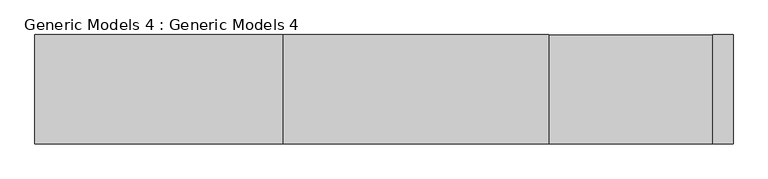
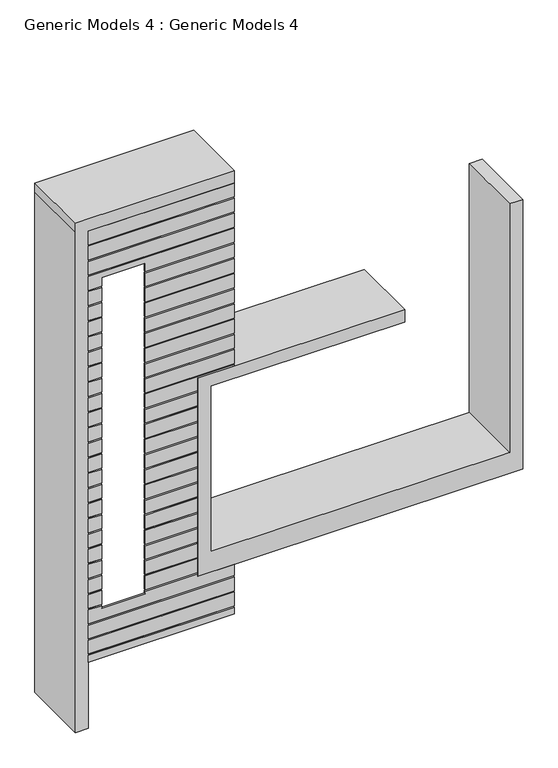
"""IFC4 building model written with IfcOpenShell, lengths in millimetres: proxy geometry, Generic Models 4 : Generic Models 4."""

from ifc_helpers import new_model, si_unit, frame, origin, place, context, project, spatial, polyline, outline, extrude, source, transform, mapped, element, save


def generic_models_4_generic_models_4_1a732ec2(model_context):
    return source(origin(), model_context, "Body", "SweptSolid", [
        extrude(outline(polyline([(-19482.368705, -12114.7027976), (-16942.368705, -12114.7027976), (-16942.368705, -12140.1027976), (-19482.368705, -12140.1027976), (-19482.368705, -12114.7027976)])), frame((0.0, 0.0, 11198.4492635), z_axis=(0.0, 0.0, 1.0), x_axis=(1.0, 0.0, 0.0)), (0.0, 0.0, 1.0), 254.0),
        extrude(outline(polyline([(-19482.368705, -12114.7027976), (-16942.368705, -12114.7027976), (-16942.368705, -12140.1027976), (-19482.368705, -12140.1027976), (-19482.368705, -12114.7027976)])), frame((0.0, 0.0, 10919.0492635), z_axis=(0.0, 0.0, 1.0), x_axis=(1.0, 0.0, 0.0)), (0.0, 0.0, 1.0), 254.0),
        extrude(outline(polyline([(-19482.368705, -12114.7027976), (-16942.368705, -12114.7027976), (-16942.368705, -12140.1027976), (-19482.368705, -12140.1027976), (-19482.368705, -12114.7027976)])), frame((0.0, 0.0, 10639.6492635), z_axis=(0.0, 0.0, 1.0), x_axis=(1.0, 0.0, 0.0)), (0.0, 0.0, 1.0), 254.0),
        extrude(outline(polyline([(10614.2492635, -19482.368705), (10360.2492635, -19482.368705), (10360.2492635, -19253.768705), (10515.6, -19253.768705), (10515.6, -18491.768705), (10360.2492635, -18491.768705), (10360.2492635, -16942.368705), (10614.2492635, -16942.368705), (10614.2492635, -19482.368705)])), frame((0.0, -12140.1027976, 0.0), z_axis=(0.0, 1.0, 0.0), x_axis=(0.0, 0.0, 1.0)), (0.0, 0.0, 1.0), 25.4),
        extrude(outline(polyline([(-18491.768705, -12114.7027976), (-16942.368705, -12114.7027976), (-16942.368705, -12140.1027976), (-18491.768705, -12140.1027976), (-18491.768705, -12114.7027976)])), frame((0.0, 0.0, 10080.8492635), z_axis=(0.0, 0.0, 1.0), x_axis=(1.0, 0.0, 0.0)), (0.0, 0.0, 1.0), 254.0),
        extrude(outline(polyline([(-19482.368705, -12114.7027976), (-19253.768705, -12114.7027976), (-19253.768705, -12140.1027976), (-19482.368705, -12140.1027976), (-19482.368705, -12114.7027976)])), frame((0.0, 0.0, 10080.8492635), z_axis=(0.0, 0.0, 1.0), x_axis=(1.0, 0.0, 0.0)), (0.0, 0.0, 1.0), 254.0),
        extrude(outline(polyline([(-18491.768705, -12114.7027976), (-16942.368705, -12114.7027976), (-16942.368705, -12140.1027976), (-18491.768705, -12140.1027976), (-18491.768705, -12114.7027976)])), frame((0.0, 0.0, 9801.4492635), z_axis=(0.0, 0.0, 1.0), x_axis=(1.0, 0.0, 0.0)), (0.0, 0.0, 1.0), 254.0),
        extrude(outline(polyline([(-19482.368705, -12114.7027976), (-19253.768705, -12114.7027976), (-19253.768705, -12140.1027976), (-19482.368705, -12140.1027976), (-19482.368705, -12114.7027976)])), frame((0.0, 0.0, 9801.4492635), z_axis=(0.0, 0.0, 1.0), x_axis=(1.0, 0.0, 0.0)), (0.0, 0.0, 1.0), 254.0),
        extrude(outline(polyline([(-18491.768705, -12114.7027976), (-16942.368705, -12114.7027976), (-16942.368705, -12140.1027976), (-18491.768705, -12140.1027976), (-18491.768705, -12114.7027976)])), frame((0.0, 0.0, 9522.0492635), z_axis=(0.0, 0.0, 1.0), x_axis=(1.0, 0.0, 0.0)), (0.0, 0.0, 1.0), 254.0),
        extrude(outline(polyline([(-19482.368705, -12114.7027976), (-19253.768705, -12114.7027976), (-19253.768705, -12140.1027976), (-19482.368705, -12140.1027976), (-19482.368705, -12114.7027976)])), frame((0.0, 0.0, 9522.0492635), z_axis=(0.0, 0.0, 1.0), x_axis=(1.0, 0.0, 0.0)), (0.0, 0.0, 1.0), 254.0),
        extrude(outline(polyline([(-18491.768705, -12114.7027976), (-16942.368705, -12114.7027976), (-16942.368705, -12140.1027976), (-18491.768705, -12140.1027976), (-18491.768705, -12114.7027976)])), frame((0.0, 0.0, 9242.6492635), z_axis=(0.0, 0.0, 1.0), x_axis=(1.0, 0.0, 0.0)), (0.0, 0.0, 1.0), 254.0),
        extrude(outline(polyline([(-19482.368705, -12114.7027976), (-19253.768705, -12114.7027976), (-19253.768705, -12140.1027976), (-19482.368705, -12140.1027976), (-19482.368705, -12114.7027976)])), frame((0.0, 0.0, 9242.6492635), z_axis=(0.0, 0.0, 1.0), x_axis=(1.0, 0.0, 0.0)), (0.0, 0.0, 1.0), 254.0),
        extrude(outline(polyline([(-18491.768705, -12114.7027976), (-16942.368705, -12114.7027976), (-16942.368705, -12140.1027976), (-18491.768705, -12140.1027976), (-18491.768705, -12114.7027976)])), frame((0.0, 0.0, 8963.2492635), z_axis=(0.0, 0.0, 1.0), x_axis=(1.0, 0.0, 0.0)), (0.0, 0.0, 1.0), 254.0),
        extrude(outline(polyline([(-19482.368705, -12114.7027976), (-19253.768705, -12114.7027976), (-19253.768705, -12140.1027976), (-19482.368705, -12140.1027976), (-19482.368705, -12114.7027976)])), frame((0.0, 0.0, 8963.2492635), z_axis=(0.0, 0.0, 1.0), x_axis=(1.0, 0.0, 0.0)), (0.0, 0.0, 1.0), 254.0),
        extrude(outline(polyline([(-18491.768705, -12114.7027976), (-16942.368705, -12114.7027976), (-16942.368705, -12140.1027976), (-18491.768705, -12140.1027976), (-18491.768705, -12114.7027976)])), frame((0.0, 0.0, 8683.8492635), z_axis=(0.0, 0.0, 1.0), x_axis=(1.0, 0.0, 0.0)), (0.0, 0.0, 1.0), 254.0),
        extrude(outline(polyline([(-19482.368705, -12114.7027976), (-19253.768705, -12114.7027976), (-19253.768705, -12140.1027976), (-19482.368705, -12140.1027976), (-19482.368705, -12114.7027976)])), frame((0.0, 0.0, 8683.8492635), z_axis=(0.0, 0.0, 1.0), x_axis=(1.0, 0.0, 0.0)), (0.0, 0.0, 1.0), 254.0),
        extrude(outline(polyline([(-18491.768705, -12114.7027976), (-16942.368705, -12114.7027976), (-16942.368705, -12140.1027976), (-18491.768705, -12140.1027976), (-18491.768705, -12114.7027976)])), frame((0.0, 0.0, 8404.4492635), z_axis=(0.0, 0.0, 1.0), x_axis=(1.0, 0.0, 0.0)), (0.0, 0.0, 1.0), 254.0),
        extrude(outline(polyline([(-19482.368705, -12114.7027976), (-19253.768705, -12114.7027976), (-19253.768705, -12140.1027976), (-19482.368705, -12140.1027976), (-19482.368705, -12114.7027976)])), frame((0.0, 0.0, 8404.4492635), z_axis=(0.0, 0.0, 1.0), x_axis=(1.0, 0.0, 0.0)), (0.0, 0.0, 1.0), 254.0),
        extrude(outline(polyline([(-18491.768705, -12114.7027976), (-16942.368705, -12114.7027976), (-16942.368705, -12140.1027976), (-18491.768705, -12140.1027976), (-18491.768705, -12114.7027976)])), frame((0.0, 0.0, 8125.0492635), z_axis=(0.0, 0.0, 1.0), x_axis=(1.0, 0.0, 0.0)), (0.0, 0.0, 1.0), 254.0),
        extrude(outline(polyline([(-19482.368705, -12114.7027976), (-19253.768705, -12114.7027976), (-19253.768705, -12140.1027976), (-19482.368705, -12140.1027976), (-19482.368705, -12114.7027976)])), frame((0.0, 0.0, 8125.0492635), z_axis=(0.0, 0.0, 1.0), x_axis=(1.0, 0.0, 0.0)), (0.0, 0.0, 1.0), 254.0),
        extrude(outline(polyline([(8099.6492635, -18491.768705), (7845.6492635, -18491.768705), (7845.6492635, -17577.368705), (8077.2, -17577.368705), (8077.2, -16942.368705), (8099.6492635, -16942.368705), (8099.6492635, -18491.768705)])), frame((0.0, -12140.1027976, 0.0), z_axis=(0.0, 1.0, 0.0), x_axis=(0.0, 0.0, 1.0)), (0.0, 0.0, 1.0), 25.4),
        extrude(outline(polyline([(-19482.368705, -12114.7027976), (-19253.768705, -12114.7027976), (-19253.768705, -12140.1027976), (-19482.368705, -12140.1027976), (-19482.368705, -12114.7027976)])), frame((0.0, 0.0, 7845.6492635), z_axis=(0.0, 0.0, 1.0), x_axis=(1.0, 0.0, 0.0)), (0.0, 0.0, 1.0), 254.0),
        extrude(outline(polyline([(-18491.768705, -12114.7027976), (-17577.368705, -12114.7027976), (-17577.368705, -12140.1027976), (-18491.768705, -12140.1027976), (-18491.768705, -12114.7027976)])), frame((0.0, 0.0, 7566.2492635), z_axis=(0.0, 0.0, 1.0), x_axis=(1.0, 0.0, 0.0)), (0.0, 0.0, 1.0), 254.0),
        extrude(outline(polyline([(-19482.368705, -12114.7027976), (-19253.768705, -12114.7027976), (-19253.768705, -12140.1027976), (-19482.368705, -12140.1027976), (-19482.368705, -12114.7027976)])), frame((0.0, 0.0, 7566.2492635), z_axis=(0.0, 0.0, 1.0), x_axis=(1.0, 0.0, 0.0)), (0.0, 0.0, 1.0), 254.0),
        extrude(outline(polyline([(-18491.768705, -12114.7027976), (-17577.368705, -12114.7027976), (-17577.368705, -12140.1027976), (-18491.768705, -12140.1027976), (-18491.768705, -12114.7027976)])), frame((0.0, 0.0, 7286.8492635), z_axis=(0.0, 0.0, 1.0), x_axis=(1.0, 0.0, 0.0)), (0.0, 0.0, 1.0), 254.0),
        extrude(outline(polyline([(-19482.368705, -12114.7027976), (-19253.768705, -12114.7027976), (-19253.768705, -12140.1027976), (-19482.368705, -12140.1027976), (-19482.368705, -12114.7027976)])), frame((0.0, 0.0, 7286.8492635), z_axis=(0.0, 0.0, 1.0), x_axis=(1.0, 0.0, 0.0)), (0.0, 0.0, 1.0), 254.0),
        extrude(outline(polyline([(-18491.768705, -12114.7027976), (-17577.368705, -12114.7027976), (-17577.368705, -12140.1027976), (-18491.768705, -12140.1027976), (-18491.768705, -12114.7027976)])), frame((0.0, 0.0, 7007.4492635), z_axis=(0.0, 0.0, 1.0), x_axis=(1.0, 0.0, 0.0)), (0.0, 0.0, 1.0), 254.0),
        extrude(outline(polyline([(-19482.368705, -12114.7027976), (-19253.768705, -12114.7027976), (-19253.768705, -12140.1027976), (-19482.368705, -12140.1027976), (-19482.368705, -12114.7027976)])), frame((0.0, 0.0, 7007.4492635), z_axis=(0.0, 0.0, 1.0), x_axis=(1.0, 0.0, 0.0)), (0.0, 0.0, 1.0), 254.0),
        extrude(outline(polyline([(-18491.768705, -12114.7027976), (-17577.368705, -12114.7027976), (-17577.368705, -12140.1027976), (-18491.768705, -12140.1027976), (-18491.768705, -12114.7027976)])), frame((0.0, 0.0, 6728.0492635), z_axis=(0.0, 0.0, 1.0), x_axis=(1.0, 0.0, 0.0)), (0.0, 0.0, 1.0), 254.0),
        extrude(outline(polyline([(-19482.368705, -12114.7027976), (-19253.768705, -12114.7027976), (-19253.768705, -12140.1027976), (-19482.368705, -12140.1027976), (-19482.368705, -12114.7027976)])), frame((0.0, 0.0, 6728.0492635), z_axis=(0.0, 0.0, 1.0), x_axis=(1.0, 0.0, 0.0)), (0.0, 0.0, 1.0), 254.0),
        extrude(outline(polyline([(-18491.768705, -12114.7027976), (-17577.368705, -12114.7027976), (-17577.368705, -12140.1027976), (-18491.768705, -12140.1027976), (-18491.768705, -12114.7027976)])), frame((0.0, 0.0, 6448.6492635), z_axis=(0.0, 0.0, 1.0), x_axis=(1.0, 0.0, 0.0)), (0.0, 0.0, 1.0), 254.0),
        extrude(outline(polyline([(-19482.368705, -12114.7027976), (-19253.768705, -12114.7027976), (-19253.768705, -12140.1027976), (-19482.368705, -12140.1027976), (-19482.368705, -12114.7027976)])), frame((0.0, 0.0, 6448.6492635), z_axis=(0.0, 0.0, 1.0), x_axis=(1.0, 0.0, 0.0)), (0.0, 0.0, 1.0), 254.0),
        extrude(outline(polyline([(-18491.768705, -12114.7027976), (-17577.368705, -12114.7027976), (-17577.368705, -12140.1027976), (-18491.768705, -12140.1027976), (-18491.768705, -12114.7027976)])), frame((0.0, 0.0, 6169.2492635), z_axis=(0.0, 0.0, 1.0), x_axis=(1.0, 0.0, 0.0)), (0.0, 0.0, 1.0), 254.0),
        extrude(outline(polyline([(-19482.368705, -12114.7027976), (-19253.768705, -12114.7027976), (-19253.768705, -12140.1027976), (-19482.368705, -12140.1027976), (-19482.368705, -12114.7027976)])), frame((0.0, 0.0, 6169.2492635), z_axis=(0.0, 0.0, 1.0), x_axis=(1.0, 0.0, 0.0)), (0.0, 0.0, 1.0), 254.0),
        extrude(outline(polyline([(-18491.768705, -12114.7027976), (-17577.368705, -12114.7027976), (-17577.368705, -12140.1027976), (-18491.768705, -12140.1027976), (-18491.768705, -12114.7027976)])), frame((0.0, 0.0, 5889.8492635), z_axis=(0.0, 0.0, 1.0), x_axis=(1.0, 0.0, 0.0)), (0.0, 0.0, 1.0), 254.0),
        extrude(outline(polyline([(-19482.368705, -12114.7027976), (-19253.768705, -12114.7027976), (-19253.768705, -12140.1027976), (-19482.368705, -12140.1027976), (-19482.368705, -12114.7027976)])), frame((0.0, 0.0, 5889.8492635), z_axis=(0.0, 0.0, 1.0), x_axis=(1.0, 0.0, 0.0)), (0.0, 0.0, 1.0), 254.0),
        extrude(outline(polyline([(-18491.768705, -12114.7027976), (-17577.368705, -12114.7027976), (-17577.368705, -12140.1027976), (-18491.768705, -12140.1027976), (-18491.768705, -12114.7027976)])), frame((0.0, 0.0, 5610.4492635), z_axis=(0.0, 0.0, 1.0), x_axis=(1.0, 0.0, 0.0)), (0.0, 0.0, 1.0), 254.0),
        extrude(outline(polyline([(-19482.368705, -12114.7027976), (-19253.768705, -12114.7027976), (-19253.768705, -12140.1027976), (-19482.368705, -12140.1027976), (-19482.368705, -12114.7027976)])), frame((0.0, 0.0, 5610.4492635), z_axis=(0.0, 0.0, 1.0), x_axis=(1.0, 0.0, 0.0)), (0.0, 0.0, 1.0), 254.0),
        extrude(outline(polyline([(-18491.768705, -12114.7027976), (-17577.368705, -12114.7027976), (-17577.368705, -12140.1027976), (-18491.768705, -12140.1027976), (-18491.768705, -12114.7027976)])), frame((0.0, 0.0, 5331.0492635), z_axis=(0.0, 0.0, 1.0), x_axis=(1.0, 0.0, 0.0)), (0.0, 0.0, 1.0), 254.0),
        extrude(outline(polyline([(-19482.368705, -12114.7027976), (-19253.768705, -12114.7027976), (-19253.768705, -12140.1027976), (-19482.368705, -12140.1027976), (-19482.368705, -12114.7027976)])), frame((0.0, 0.0, 5331.0492635), z_axis=(0.0, 0.0, 1.0), x_axis=(1.0, 0.0, 0.0)), (0.0, 0.0, 1.0), 254.0),
        extrude(outline(polyline([(-18491.768705, -12114.7027976), (-17577.368705, -12114.7027976), (-17577.368705, -12140.1027976), (-18491.768705, -12140.1027976), (-18491.768705, -12114.7027976)])), frame((0.0, 0.0, 5051.6492635), z_axis=(0.0, 0.0, 1.0), x_axis=(1.0, 0.0, 0.0)), (0.0, 0.0, 1.0), 254.0),
        extrude(outline(polyline([(-19482.368705, -12114.7027976), (-19253.768705, -12114.7027976), (-19253.768705, -12140.1027976), (-19482.368705, -12140.1027976), (-19482.368705, -12114.7027976)])), frame((0.0, 0.0, 5051.6492635), z_axis=(0.0, 0.0, 1.0), x_axis=(1.0, 0.0, 0.0)), (0.0, 0.0, 1.0), 254.0),
        extrude(outline(polyline([(-18491.768705, -12114.7027976), (-17577.368705, -12114.7027976), (-17577.368705, -12140.1027976), (-18491.768705, -12140.1027976), (-18491.768705, -12114.7027976)])), frame((0.0, 0.0, 4772.2492635), z_axis=(0.0, 0.0, 1.0), x_axis=(1.0, 0.0, 0.0)), (0.0, 0.0, 1.0), 254.0),
        extrude(outline(polyline([(-19482.368705, -12114.7027976), (-19253.768705, -12114.7027976), (-19253.768705, -12140.1027976), (-19482.368705, -12140.1027976), (-19482.368705, -12114.7027976)])), frame((0.0, 0.0, 4772.2492635), z_axis=(0.0, 0.0, 1.0), x_axis=(1.0, 0.0, 0.0)), (0.0, 0.0, 1.0), 254.0),
        extrude(outline(polyline([(-18491.768705, -12114.7027976), (-17577.368705, -12114.7027976), (-17577.368705, -12140.1027976), (-18491.768705, -12140.1027976), (-18491.768705, -12114.7027976)])), frame((0.0, 0.0, 4492.8492635), z_axis=(0.0, 0.0, 1.0), x_axis=(1.0, 0.0, 0.0)), (0.0, 0.0, 1.0), 254.0),
        extrude(outline(polyline([(-19482.368705, -12114.7027976), (-19253.768705, -12114.7027976), (-19253.768705, -12140.1027976), (-19482.368705, -12140.1027976), (-19482.368705, -12114.7027976)])), frame((0.0, 0.0, 4492.8492635), z_axis=(0.0, 0.0, 1.0), x_axis=(1.0, 0.0, 0.0)), (0.0, 0.0, 1.0), 254.0),
        extrude(outline(polyline([(4467.4492635, -18491.768705), (4419.6, -18491.768705), (4419.6, -19253.768705), (4467.4492635, -19253.768705), (4467.4492635, -19482.368705), (4213.4492635, -19482.368705), (4213.4492635, -16942.368705), (4419.6, -16942.368705), (4419.6, -17577.368705), (4467.4492635, -17577.368705), (4467.4492635, -18491.768705)])), frame((0.0, -12140.1027976, 0.0), z_axis=(0.0, 1.0, 0.0), x_axis=(0.0, 0.0, 1.0)), (0.0, 0.0, 1.0), 25.4),
        extrude(outline(polyline([(-19482.368705, -12114.7027976), (-16942.368705, -12114.7027976), (-16942.368705, -12140.1027976), (-19482.368705, -12140.1027976), (-19482.368705, -12114.7027976)])), frame((0.0, 0.0, 3934.0492635), z_axis=(0.0, 0.0, 1.0), x_axis=(1.0, 0.0, 0.0)), (0.0, 0.0, 1.0), 254.0),
        extrude(outline(polyline([(-19482.368705, -12114.7027976), (-16942.368705, -12114.7027976), (-16942.368705, -12140.1027976), (-19482.368705, -12140.1027976), (-19482.368705, -12114.7027976)])), frame((0.0, 0.0, 3654.6492635), z_axis=(0.0, 0.0, 1.0), x_axis=(1.0, 0.0, 0.0)), (0.0, 0.0, 1.0), 254.0),
        extrude(outline(polyline([(-19482.368705, -12114.7027976), (-16942.368705, -12114.7027976), (-16942.368705, -12140.1027976), (-19482.368705, -12140.1027976), (-19482.368705, -12114.7027976)])), frame((0.0, 0.0, 3505.2), z_axis=(0.0, 0.0, 1.0), x_axis=(1.0, 0.0, 0.0)), (0.0, 0.0, 1.0), 124.0492635),
        extrude(outline(polyline([(4419.6, -11913.168705), (4800.6, -11913.168705), (9386.2446878, -11913.168705), (9386.2446878, -12141.768705), (4800.6, -12141.768705), (4800.6, -17348.768705), (7848.6, -17348.768705), (7848.6, -13970.568705), (8077.2, -13970.568705), (8077.2, -17577.368705), (7848.6, -17577.368705), (4800.6, -17577.368705), (4419.6, -17577.368705), (4419.6, -11913.168705)])), frame((0.0, -12140.1027976, 0.0), z_axis=(0.0, 1.0, 0.0), x_axis=(0.0, 0.0, 1.0)), (0.0, 0.0, 1.0), 1219.2),
        extrude(outline(polyline([(11452.4492635, -19482.368705), (11452.4492635, -16942.368705), (11681.0492635, -16942.368705), (11681.0492635, -19710.968705), (11506.2, -19710.968705), (2286.0, -19710.968705), (2286.0, -19482.368705), (11452.4492635, -19482.368705)])), frame((0.0, -12140.1027976, 0.0), z_axis=(0.0, 1.0, 0.0), x_axis=(0.0, 0.0, 1.0)), (0.0, 0.0, 1.0), 1219.2),
    ])


if __name__ == "__main__":
    model = new_model("IFC4")
    model_context = context("Model", 3, world=origin())
    ifc_project = project(units=[si_unit("LENGTHUNIT", "METRE", prefix="MILLI")], contexts=[model_context])
    site = spatial("IfcSite", under=ifc_project)
    building = spatial("IfcBuilding", under=site)
    placement = place(None, origin())
    generic_models_4_generic_models_4_shape = generic_models_4_generic_models_4_1a732ec2(model_context)
    element("IfcBuildingElementProxy", 1, Name="Generic Models 4 : Generic Models 4", ObjectType="Generic Models 4 : Generic Models 4", at=placement, inside=building, context=model_context, shape_type="MappedRepresentation", body=[
        mapped(generic_models_4_generic_models_4_shape, transform((0.0, 0.0, 0.0), x_axis=(1.0, 0.0, 0.0), y_axis=(0.0, 1.0, 0.0), z_axis=(0.0, 0.0, 1.0))),
    ])
    save(model, "model.ifc")

# Revit data of these elements
# Element 1 (IfcBuildingElementProxy, "Generic Models 4 : Generic Models 4")
#   Materials on its faces: "Softwood, Lumber", "Gypsum Wall Board"
# Materials
#   "Softwood, Lumber": class "Wood", colour RGB 223 192 134, transparency 0, Description = "Pinus Echinata", Cost = 0
#   "Gypsum Wall Board": class "Generic", colour RGB 228 228 228, transparency 0, Description = "Gypsum Wall Board", Cost = 0
